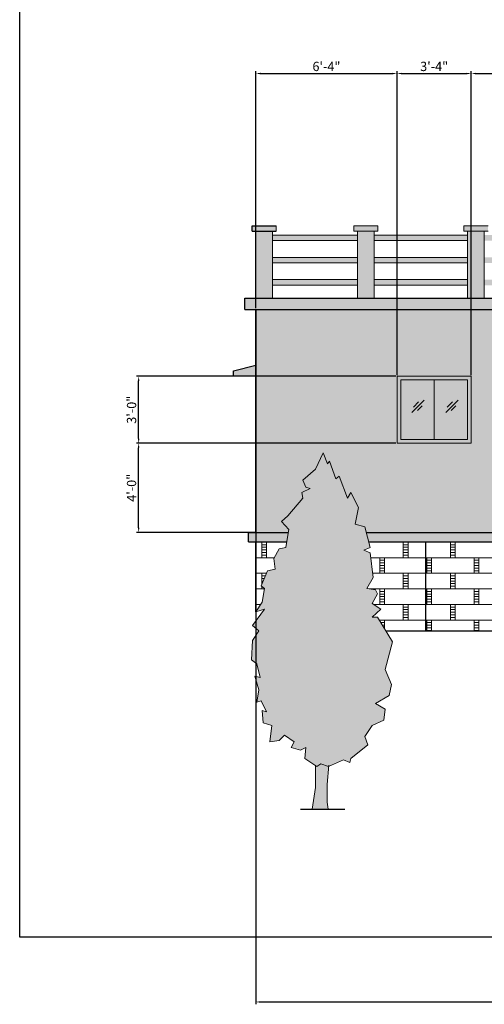
# Model space of a CAD drawing. Units: inches. Extents: x 1662 to 23131, y 1265 to 19127.
# Tile 21 of 26: x 21861 to 22111, y 17831 to 18361. Entities that reach past the tile are written whole.
import ezdxf

# ---------------------------------------------------------------- set-up
doc = ezdxf.new("R2010")
doc.units = ezdxf.units.IN
for name, color, linetype, lineweight in [('A-ANNO-DIMS', 4, 'Continuous', 18), ('A-ANNO-TTLB', 7, 'Continuous', 25), ('A-ELEV', 7, 'Continuous', 25), ('A-ELEV-GLAZ', 4, 'Continuous', 18), ('A-ELEV-PATT', 8, 'Continuous', 13), ('A-ELEV-RAIL', 7, 'Continuous', 18), ('A-ELEV-SURF-PATT', 252, 'Continuous', 13), ('L-PLNT', 3, 'Continuous', 18)]:
    doc.layers.add(name, color=color, linetype=linetype, lineweight=lineweight)
doc.styles.get("Standard").update_dxf_attribs({"font": 'arial.ttf'})
doc.dimstyles.new('ISO-25', dxfattribs={"dimtxt": 5, "dimasz": 2.5, "dimexe": 1.25, "dimexo": 0.625, "dimtad": 1, "dimlunit": 3, "dimtxsty": 'Standard', "dimcen": 2.5, "dimadec": 0, "dimazin": 0, "dimtfac": 1, "dimtmove": 0, "dimatfit": 3, "dimfxl": 1, "dimarcsym": 0})

# ---------------------------------------------------------------- blocks, each defined once
blk = doc.blocks.new('*U136')
blk.add_lwpolyline([(-69.9516, 4869.1546), (-172.212, 4644.4154), (-347.5228, 4494.6062), (-303.6824, 4400.9564), (-245.2624, 4382.2366), (-362.1278, 4326.0518), (-347.5228, 4251.1472), (-552.0182, 4007.6882), (-639.6736, 3932.7836), (-537.4132, 3820.414), (-552.0182, 3745.5094), (-581.2536, 3576.955), (-668.8836, 3558.2098), (-741.934, 3427.1204), (-727.329, 3277.3112), (-829.5894, 3258.5914), (-917.2194, 3052.572), (-873.4044, 3015.1324), (-902.6144, 2827.8582), (-990.2698, 2696.7434), (-873.4044, 2734.2084), (-1034.0848, 2509.4692), (-946.4294, 2434.5646), (-1034.0848, 2303.4752), (-1048.6898, 2041.2964), (-975.6648, 1985.1116), (-931.8244, 1797.8374), (-1004.8748, 1816.5572), (-946.4294, 1629.283), (-975.6648, 1460.7286), (-917.2194, 1479.4738), (-844.1944, 1329.6392), (-902.6144, 1348.3844), (-888.0094, 1179.83), (-771.144, 1142.365), (-800.354, 917.6512), (-668.8836, 936.371), (-595.8586, 1011.2756), (-464.3882, 917.6512), (-508.2032, 842.7212), (-376.7328, 805.2816), (-303.6824, 842.7212), (-318.2874, 692.912), (-157.607, 580.5424), (-99.187, 618.0074), (3.0734, 580.5424), (207.5942, 674.1922), (295.2496, 636.7272), (309.8546, 692.912), (543.56, 880.1862), (499.745, 992.5558), (602.0054, 1142.365), (762.6858, 1217.2696), (777.2908, 1367.1042), (645.8204, 1442.0088), (835.7362, 1554.3784), (864.9462, 1704.1876), (777.2908, 1910.207), (879.5512, 2284.7554), (675.0304, 2621.8388), (602.0054, 2621.8388), (718.8708, 2734.2084), (602.0054, 2809.113), (675.0304, 2940.2024), (645.8204, 2996.3872), (528.955, 3015.1324), (616.6104, 3164.9416), (572.7954, 3502.0504), (485.14, 3539.49), (572.7954, 3576.955), (499.745, 3857.8536), (368.2746, 3895.3186), (412.0896, 4120.0578), (309.8546, 4326.0518), (266.0142, 4251.1472), (149.1488, 4550.791), (105.3338, 4513.326), (17.6784, 4756.785), (-11.5316, 4719.32)], close=True)
for points in [[(-173.0502, 601.1926), (-173.0502, 296.3926), (-219.1258, 0)], [(9.8298, 601.1926), (-14.6304, 337.0834), (-14.6304, 93.6244), (0, 0)]]:
    blk.add_lwpolyline(points)
blk = doc.blocks.new('GLAZ-REFLECTION')
for p, q in [((0, 0), (6.63, 6.69)), ((0.83, 2.91), (3.6, 5.77)), ((2.93, 0.98), (5.5, 3.58))]:
    blk.add_line(p, q)
blk = doc.blocks.new('*D257')
at = {"layer": 'A-ANNO-DIMS', "color": 0, "lineweight": -2, "transparency": 16777216}
for p, q in [((21988.15, 18204.6), (21988.15, 17831.29)), ((22540.15, 18204.6), (22540.15, 17831.29)), ((21990.65, 17832.54), (22537.65, 17832.54))]:
    blk.add_line(p, q, dxfattribs=at)
at = {"layer": 'A-ANNO-DIMS', "color": 0, "transparency": 16777216}
for points in [[(21990.65, 17832.96), (21990.65, 17832.12), (21988.15, 17832.54)], [(22537.65, 17832.96), (22537.65, 17832.12), (22540.15, 17832.54)]]:
    blk.add_solid(points, dxfattribs=at)
at = {"layer": 'Defpoints', "color": 0, "transparency": 16777216}
for p in [(21988.15, 18205.22), (22540.15, 18205.22), (22540.15, 17832.54)]:
    blk.add_point(p, dxfattribs=at)
at = {"layer": 'A-ANNO-DIMS', "color": 0, "transparency": 16777216, "insert": (22264.15, 17835.72), "char_height": 5, "attachment_point": 5}
blk.add_mtext('46\'-0"', dxfattribs=at)
blk = doc.blocks.new('*D259')
at = {"layer": 'A-ANNO-DIMS', "color": 0, "lineweight": -2, "transparency": 16777216}
for p, q in [((21988.15, 18205.85), (21988.15, 18333.37)), ((21990.65, 18332.12), (22061.65, 18332.12)), ((22064.15, 18169.85), (22064.15, 18333.37))]:
    blk.add_line(p, q, dxfattribs=at)
at = {"layer": 'A-ANNO-DIMS', "color": 0, "transparency": 16777216}
for points in [[(21990.65, 18332.54), (21990.65, 18331.71), (21988.15, 18332.12)], [(22061.65, 18332.54), (22061.65, 18331.71), (22064.15, 18332.12)]]:
    blk.add_solid(points, dxfattribs=at)
at = {"layer": 'Defpoints', "color": 0, "transparency": 16777216}
for p in [(22064.15, 18332.12), (21988.15, 18205.22), (22064.15, 18169.22)]:
    blk.add_point(p, dxfattribs=at)
at = {"layer": 'A-ANNO-DIMS', "color": 0, "transparency": 16777216, "insert": (22026.15, 18335.3), "char_height": 5, "attachment_point": 5}
blk.add_mtext('6\'-4"', dxfattribs=at)
blk = doc.blocks.new('*D260')
at = {"layer": 'A-ANNO-DIMS', "color": 0, "lineweight": -2, "transparency": 16777216}
for p, q in [((22064.15, 18169.85), (22064.15, 18333.37)), ((22066.65, 18332.12), (22101.65, 18332.12)), ((22104.15, 18169.85), (22104.15, 18333.37))]:
    blk.add_line(p, q, dxfattribs=at)
at = {"layer": 'A-ANNO-DIMS', "color": 0, "transparency": 16777216}
for points in [[(22066.65, 18332.54), (22066.65, 18331.71), (22064.15, 18332.12)], [(22101.65, 18332.54), (22101.65, 18331.71), (22104.15, 18332.12)]]:
    blk.add_solid(points, dxfattribs=at)
at = {"layer": 'Defpoints', "color": 0, "transparency": 16777216}
for p in [(22104.15, 18332.12), (22064.15, 18169.22), (22104.15, 18169.22)]:
    blk.add_point(p, dxfattribs=at)
at = {"layer": 'A-ANNO-DIMS', "color": 0, "transparency": 16777216, "insert": (22084.15, 18335.3), "char_height": 5, "attachment_point": 5}
blk.add_mtext('3\'-4"', dxfattribs=at)
blk = doc.blocks.new('*D261')
at = {"layer": 'A-ANNO-DIMS', "color": 0, "lineweight": -2, "transparency": 16777216}
for p, q in [((22104.15, 18169.85), (22104.15, 18333.37)), ((22106.65, 18332.12), (22168.65, 18332.12)), ((22171.15, 18169.85), (22171.15, 18333.37))]:
    blk.add_line(p, q, dxfattribs=at)
at = {"layer": 'A-ANNO-DIMS', "color": 0, "transparency": 16777216}
for points in [[(22106.65, 18332.54), (22106.65, 18331.71), (22104.15, 18332.12)], [(22168.65, 18332.54), (22168.65, 18331.71), (22171.15, 18332.12)]]:
    blk.add_solid(points, dxfattribs=at)
at = {"layer": 'Defpoints', "color": 0, "transparency": 16777216}
for p in [(22171.15, 18332.12), (22104.15, 18169.22), (22171.15, 18169.22)]:
    blk.add_point(p, dxfattribs=at)
at = {"layer": 'A-ANNO-DIMS', "color": 0, "transparency": 16777216, "insert": (22137.65, 18335.29), "char_height": 5, "attachment_point": 5}
blk.add_mtext('5\'-7"', dxfattribs=at)
blk = doc.blocks.new('*D266')
at = {"layer": 'A-ANNO-DIMS', "color": 0, "lineweight": -2, "transparency": 16777216}
for p, q in [((22063.52, 18169.22), (21923.8, 18169.22)), ((21925.05, 18135.72), (21925.05, 18166.72)), ((22063.52, 18133.22), (21923.8, 18133.22))]:
    blk.add_line(p, q, dxfattribs=at)
at = {"layer": 'A-ANNO-DIMS', "color": 0, "transparency": 16777216}
for points in [[(21924.63, 18166.72), (21925.47, 18166.72), (21925.05, 18169.22)], [(21924.63, 18135.72), (21925.47, 18135.72), (21925.05, 18133.22)]]:
    blk.add_solid(points, dxfattribs=at)
at = {"layer": 'Defpoints', "color": 0, "transparency": 16777216}
for p in [(21925.05, 18169.22), (22064.15, 18169.22), (22064.15, 18133.22)]:
    blk.add_point(p, dxfattribs=at)
at = {"layer": 'A-ANNO-DIMS', "color": 0, "transparency": 16777216, "insert": (21921.87, 18151.22), "char_height": 5, "attachment_point": 5, "rotation": 90}
blk.add_mtext('3\'-0"', dxfattribs=at)
blk = doc.blocks.new('*D267')
at = {"layer": 'A-ANNO-DIMS', "color": 0, "lineweight": -2, "transparency": 16777216}
for p, q in [((22063.52, 18133.22), (21923.8, 18133.22)), ((21925.05, 18087.72), (21925.05, 18130.72)), ((21987.52, 18085.22), (21923.8, 18085.22))]:
    blk.add_line(p, q, dxfattribs=at)
at = {"layer": 'A-ANNO-DIMS', "color": 0, "transparency": 16777216}
for points in [[(21924.63, 18130.72), (21925.47, 18130.72), (21925.05, 18133.22)], [(21924.63, 18087.72), (21925.47, 18087.72), (21925.05, 18085.22)]]:
    blk.add_solid(points, dxfattribs=at)
at = {"layer": 'Defpoints', "color": 0, "transparency": 16777216}
for p in [(21925.05, 18133.22), (22064.15, 18133.22), (21988.15, 18085.22)]:
    blk.add_point(p, dxfattribs=at)
at = {"layer": 'A-ANNO-DIMS', "color": 0, "transparency": 16777216, "insert": (21921.87, 18109.22), "char_height": 5, "attachment_point": 5, "rotation": 90}
blk.add_mtext('4\'-0"', dxfattribs=at)

msp = doc.modelspace()

# ---------------------------------------------------------------- hatches: boundary and pattern name
at = {"layer": 'A-ELEV-PATT'}
h = msp.add_hatch(dxfattribs=at)
h.set_pattern_fill('BRSTONE', color=256)
h.paths.add_polyline_path([(22156.149, 18080.223), (22079.649, 18080.223), (22079.649, 18032.223), (22156.149, 18032.223)])
h.paths.add_polyline_path([(22079.649, 18080.223), (22048.849, 18080.223), (22049.648, 18077.151), (22046.197, 18075.676), (22049.648, 18074.202), (22051.373, 18060.93), (22047.922, 18055.032), (22052.523, 18054.294), (22053.673, 18052.082), (22050.798, 18046.921), (22055.399, 18043.972), (22050.798, 18039.548), (22053.673, 18039.548), (22058.118, 18032.223), (22079.649, 18032.223)])
h.paths.add_polyline_path([(21997.887, 18071.252), (22000.763, 18076.413), (22004.213, 18077.151), (22004.746, 18080.223), (21988.149, 18080.223), (21988.149, 18042.556), (21991.561, 18047.659), (21992.711, 18055.032), (21990.986, 18056.506), (21994.436, 18064.617), (21998.462, 18065.354)])
at = {"layer": 'A-ELEV-SURF-PATT'}
h = msp.add_hatch(color=256, dxfattribs=at)
h.dxf.hatch_style = 1
h.paths.add_polyline_path([(22225.149, 18211.223), (21982.149, 18211.223), (21982.149, 18205.223), (22225.149, 18205.223)])
h.paths.add_polyline_path([(22546.149, 18211.223), (22339.149, 18211.223), (22339.149, 18205.223), (22546.149, 18205.223)])
h.paths.add_polyline_path([(22351.149, 18300.223), (22213.149, 18300.223), (22213.149, 18295.223), (22351.149, 18295.223)])
h = msp.add_hatch(color=256, dxfattribs=at)
h.dxf.hatch_style = 1
h.paths.add_polyline_path([(22225.149, 18205.223), (21988.149, 18205.223), (21988.149, 18085.223), (22005.644, 18085.223), (22005.939, 18086.736), (22001.913, 18091.16), (22005.364, 18094.109), (22013.415, 18103.694), (22012.84, 18106.643), (22017.441, 18108.855), (22015.141, 18109.592), (22013.415, 18113.279), (22020.317, 18119.177), (22024.343, 18128.025), (22026.643, 18122.126), (22027.793, 18123.601), (22031.244, 18114.016), (22032.969, 18115.491), (22037.57, 18103.694), (22039.296, 18106.643), (22043.321, 18098.533), (22041.596, 18089.685), (22046.772, 18088.21), (22047.549, 18085.223), (22171.149, 18085.223), (22171.149, 18169.223), (22213.149, 18169.223), (22213.149, 18085.223), (22225.149, 18085.223)])
h.paths.add_polyline_path([(22064.149, 18169.223), (22104.149, 18169.223), (22104.149, 18133.223), (22064.149, 18133.223)], flags=16)
h.paths.add_polyline_path([(22066.149, 18167.223), (22102.149, 18167.223), (22102.149, 18135.223), (22066.149, 18135.223)], flags=0)
h.paths.add_polyline_path([(22540.149, 18205.223), (22339.149, 18205.223), (22339.149, 18085.223), (22540.149, 18085.223)])
h.paths.add_polyline_path([(22415.149, 18169.223), (22455.149, 18169.223), (22455.149, 18133.223), (22415.149, 18133.223)], flags=16)
h.paths.add_polyline_path([(22417.149, 18167.223), (22453.149, 18167.223), (22453.149, 18135.223), (22417.149, 18135.223)], flags=0)
h.paths.add_polyline_path([(22339.149, 18205.223), (22339.149, 18268.223), (22252.149, 18268.223), (22252.149, 18211.223), (22252.149, 18085.223), (22339.149, 18085.223)], flags=17)
h.paths.add_polyline_path([(22272.061, 18145.984), (22272.061, 18250.207), (22312.36, 18250.207), (22312.36, 18145.984)], flags=16)
h.paths.add_polyline_path([(22275.061, 18148.984), (22275.061, 18247.207), (22309.36, 18247.207), (22309.36, 18148.984)], flags=0)
h.paths.add_polyline_path([(22243.149, 18211.223), (22243.149, 18277.223), (22339.149, 18277.223), (22339.149, 18295.223), (22225.149, 18295.223), (22225.149, 18211.223), (22225.149, 18085.223), (22243.149, 18085.223)])
h = msp.add_hatch(color=256, dxfattribs=at)
h.dxf.hatch_style = 1
h.paths.add_polyline_path([(21999.149, 18250.223), (21986.149, 18250.223), (21986.149, 18247.223), (21999.149, 18247.223)])
h.paths.add_polyline_path([(22053.899, 18250.223), (22040.899, 18250.223), (22040.899, 18247.223), (22053.899, 18247.223)])
h.paths.add_polyline_path([(22113.149, 18250.223), (22100.149, 18250.223), (22100.149, 18247.223), (22113.149, 18247.223)])
h.paths.add_polyline_path([(22172.399, 18250.223), (22159.399, 18250.223), (22159.399, 18247.223), (22172.399, 18247.223)])
h.paths.add_polyline_path([(22363.649, 18250.223), (22350.649, 18250.223), (22350.649, 18247.223), (22363.649, 18247.223)])
h.paths.add_polyline_path([(22436.399, 18250.223), (22423.399, 18250.223), (22423.399, 18247.223), (22436.399, 18247.223)])
h.paths.add_polyline_path([(22495.649, 18250.223), (22482.649, 18250.223), (22482.649, 18247.223), (22495.649, 18247.223)])
h.paths.add_polyline_path([(22542.149, 18250.223), (22529.149, 18250.223), (22529.149, 18247.223), (22542.149, 18247.223)])
h = msp.add_hatch(color=256, dxfattribs=at)
h.dxf.hatch_style = 1
h.paths.add_polyline_path([(22493.649, 18247.223), (22484.649, 18247.223), (22484.649, 18211.223), (22493.649, 18211.223)])
h.paths.add_polyline_path([(22434.399, 18247.223), (22425.399, 18247.223), (22425.399, 18211.223), (22434.399, 18211.223)])
h.paths.add_polyline_path([(22361.649, 18247.223), (22352.649, 18247.223), (22352.649, 18211.223), (22361.649, 18211.223)])
h.paths.add_polyline_path([(22170.399, 18247.223), (22161.399, 18247.223), (22161.399, 18211.223), (22170.399, 18211.223)])
h.paths.add_polyline_path([(22111.149, 18247.223), (22102.149, 18247.223), (22102.149, 18211.223), (22111.149, 18211.223)])
h.paths.add_polyline_path([(22051.899, 18247.223), (22042.899, 18247.223), (22042.899, 18211.223), (22051.899, 18211.223)])
h.paths.add_polyline_path([(21997.149, 18247.223), (21988.149, 18247.223), (21988.149, 18211.223), (21997.149, 18211.223)])
h = msp.add_hatch(color=256, dxfattribs=at)
h.dxf.hatch_style = 1
h.paths.add_polyline_path([(22104.149, 18169.223), (22064.149, 18169.223), (22064.149, 18133.223), (22104.149, 18133.223)])
h.paths.add_polyline_path([(22102.149, 18167.223), (22102.149, 18135.223), (22066.149, 18135.223), (22066.149, 18167.223)], flags=16)
h.paths.add_polyline_path([(22455.149, 18169.223), (22415.149, 18169.223), (22415.149, 18133.223), (22455.149, 18133.223)])
h.paths.add_polyline_path([(22453.149, 18167.223), (22453.149, 18135.223), (22417.149, 18135.223), (22417.149, 18167.223)], flags=16)
h.paths.add_polyline_path([(22312.36, 18250.207), (22272.061, 18250.207), (22272.061, 18145.984), (22312.36, 18145.984)])
h.paths.add_polyline_path([(22309.36, 18148.984), (22275.061, 18148.984), (22275.061, 18247.207), (22309.36, 18247.207)], flags=16)
h.paths.add_polyline_path([(22042.899, 18245.223), (21997.149, 18245.223), (21997.149, 18242.223), (22042.899, 18242.223)])
h.paths.add_polyline_path([(22042.899, 18233.223), (21997.149, 18233.223), (21997.149, 18230.223), (22042.899, 18230.223)])
h.paths.add_polyline_path([(22042.899, 18221.223), (21997.149, 18221.223), (21997.149, 18218.223), (22042.899, 18218.223)])
h.paths.add_polyline_path([(22102.149, 18221.223), (22051.899, 18221.223), (22051.899, 18218.223), (22102.149, 18218.223)])
h.paths.add_polyline_path([(22102.149, 18233.223), (22051.899, 18233.223), (22051.899, 18230.223), (22102.149, 18230.223)])
h.paths.add_polyline_path([(22102.149, 18245.223), (22051.899, 18245.223), (22051.899, 18242.223), (22102.149, 18242.223)])
h.paths.add_polyline_path([(22161.399, 18245.223), (22111.149, 18245.223), (22111.149, 18242.223), (22161.399, 18242.223)])
h.paths.add_polyline_path([(22161.399, 18233.223), (22111.149, 18233.223), (22111.149, 18230.223), (22161.399, 18230.223)])
h.paths.add_polyline_path([(22161.399, 18221.223), (22111.149, 18221.223), (22111.149, 18218.223), (22161.399, 18218.223)])
h.paths.add_polyline_path([(22225.149, 18221.223), (22170.399, 18221.223), (22170.399, 18218.223), (22225.149, 18218.223)])
h.paths.add_polyline_path([(22225.149, 18233.223), (22170.399, 18233.223), (22170.399, 18230.223), (22225.149, 18230.223)])
h.paths.add_polyline_path([(22225.149, 18245.223), (22170.399, 18245.223), (22170.399, 18242.223), (22225.149, 18242.223)])
h.paths.add_polyline_path([(22352.649, 18233.223), (22339.149, 18233.223), (22339.149, 18230.223), (22352.649, 18230.223)])
h.paths.add_polyline_path([(22352.649, 18221.223), (22339.149, 18221.223), (22339.149, 18218.223), (22352.649, 18218.223)])
h.paths.add_polyline_path([(22352.649, 18245.223), (22339.149, 18245.223), (22339.149, 18242.223), (22352.649, 18242.223)])
h.paths.add_polyline_path([(22425.399, 18245.223), (22361.649, 18245.223), (22361.649, 18242.223), (22425.399, 18242.223)])
h.paths.add_polyline_path([(22425.399, 18233.223), (22361.649, 18233.223), (22361.649, 18230.223), (22425.399, 18230.223)])
h.paths.add_polyline_path([(22425.399, 18221.223), (22361.649, 18221.223), (22361.649, 18218.223), (22425.399, 18218.223)])
h.paths.add_polyline_path([(22484.649, 18245.223), (22434.399, 18245.223), (22434.399, 18242.223), (22484.649, 18242.223)])
h.paths.add_polyline_path([(22484.649, 18233.223), (22434.399, 18233.223), (22434.399, 18230.223), (22484.649, 18230.223)])
h.paths.add_polyline_path([(22484.649, 18221.223), (22434.399, 18221.223), (22434.399, 18218.223), (22484.649, 18218.223)])
h.paths.add_polyline_path([(22531.149, 18221.223), (22493.649, 18221.223), (22493.649, 18218.223), (22531.149, 18218.223)])
h.paths.add_polyline_path([(22531.149, 18233.223), (22493.649, 18233.223), (22493.649, 18230.223), (22531.149, 18230.223)])
h.paths.add_polyline_path([(22531.149, 18245.223), (22493.649, 18245.223), (22493.649, 18242.223), (22531.149, 18242.223)])
h = msp.add_hatch(color=256, dxfattribs=at)
h.dxf.hatch_style = 1
h.paths.add_polyline_path([(21988.149, 18175.223), (21976.149, 18172.223), (21976.149, 18169.223), (21988.149, 18169.223)])
h = msp.add_hatch(color=256, dxfattribs=at)
h.dxf.hatch_style = 1
h.paths.add_polyline_path([(22084.149, 18167.223), (22066.149, 18167.223), (22066.149, 18135.223), (22084.149, 18135.223)])
h.paths.add_polyline_path([(22102.149, 18167.223), (22084.149, 18167.223), (22084.149, 18135.223), (22102.149, 18135.223)])
h.paths.add_polyline_path([(22435.149, 18167.223), (22417.149, 18167.223), (22417.149, 18135.223), (22435.149, 18135.223)])
h.paths.add_polyline_path([(22453.149, 18167.223), (22435.149, 18167.223), (22435.149, 18135.223), (22453.149, 18135.223)])
h = msp.add_hatch(color=256, dxfattribs=at)
h.dxf.hatch_style = 1
h.paths.add_polyline_path([(22053.673, 18039.548), (22050.798, 18039.548), (22055.399, 18043.972), (22050.798, 18046.921), (22053.673, 18052.082), (22052.523, 18054.294), (22047.922, 18055.032), (22051.373, 18060.93), (22049.648, 18074.202), (22046.197, 18075.676), (22049.648, 18077.151), (22046.772, 18088.21), (22041.596, 18089.685), (22043.321, 18098.533), (22039.296, 18106.643), (22037.57, 18103.694), (22032.969, 18115.491), (22031.244, 18114.016), (22027.793, 18123.601), (22026.643, 18122.126), (22024.343, 18128.025), (22020.317, 18119.177), (22013.415, 18113.279), (22015.141, 18109.592), (22017.441, 18108.855), (22012.84, 18106.643), (22013.415, 18103.694), (22005.364, 18094.109), (22001.913, 18091.16), (22005.939, 18086.736), (22005.364, 18083.787), (22004.213, 18077.151), (22000.763, 18076.413), (21997.887, 18071.252), (21998.462, 18065.354), (21994.436, 18064.617), (21990.986, 18056.506), (21992.711, 18055.032), (21991.561, 18047.659), (21988.149, 18042.556), (21988.149, 18042.51), (21992.711, 18043.972), (21986.385, 18035.124), (21989.836, 18032.175), (21986.385, 18027.014), (21985.81, 18016.692), (21988.685, 18014.48), (21990.411, 18007.107), (21987.535, 18007.844), (21989.836, 18000.471), (21988.685, 17993.835), (21990.986, 17994.573), (21993.861, 17988.674), (21991.561, 17989.412), (21992.136, 17982.776), (21996.737, 17981.301), (21995.587, 17972.454), (22000.763, 17973.191), (22003.638, 17976.14), (22008.814, 17972.454), (22007.089, 17969.504), (22012.265, 17968.03), (22015.141, 17969.504), (22014.566, 17963.606), (22020.892, 17959.182), (22023.192, 17960.657), (22027.218, 17959.182), (22035.27, 17962.869), (22038.721, 17961.394), (22039.296, 17963.606), (22048.497, 17970.979), (22046.772, 17975.403), (22050.798, 17981.301), (22057.124, 17984.25), (22057.699, 17990.149), (22052.523, 17993.098), (22060, 17997.522), (22061.15, 18003.42), (22057.699, 18011.531), (22061.725, 18026.277)], flags=17)
h.paths.add_polyline_path([(22061.725, 18026.277), (22053.673, 18039.548), (22050.798, 18039.548), (22055.399, 18043.972), (22050.798, 18046.921), (22053.673, 18052.082), (22052.523, 18054.294), (22047.922, 18055.032), (22051.373, 18060.93), (22049.648, 18074.202), (22046.197, 18075.676), (22049.648, 18077.151), (22046.772, 18088.21), (22041.596, 18089.685), (22043.321, 18098.533), (22039.296, 18106.643), (22037.57, 18103.694), (22032.969, 18115.491), (22031.244, 18114.016), (22027.793, 18123.601), (22026.643, 18122.126), (22024.343, 18128.025), (22020.317, 18119.177), (22013.415, 18113.279), (22015.141, 18109.592), (22017.441, 18108.855), (22012.84, 18106.643), (22013.415, 18103.694), (22005.364, 18094.109), (22001.913, 18091.16), (22005.939, 18086.736), (22005.364, 18083.787), (22004.213, 18077.151), (22000.763, 18076.413), (21997.887, 18071.252), (21998.462, 18065.354), (21994.436, 18064.617), (21990.986, 18056.506), (21992.711, 18055.032), (21991.561, 18047.659), (21988.11, 18042.497), (21992.711, 18043.972), (21986.385, 18035.124), (21989.836, 18032.175), (21986.385, 18027.014), (21985.81, 18016.692), (21988.685, 18014.48), (21990.411, 18007.107), (21987.535, 18007.844), (21989.836, 18000.471), (21988.685, 17993.835), (21990.986, 17994.573), (21993.861, 17988.674), (21991.561, 17989.412), (21992.136, 17982.776), (21996.737, 17981.301), (21995.587, 17972.454), (22000.763, 17973.191), (22003.638, 17976.14), (22008.814, 17972.454), (22007.089, 17969.504), (22012.265, 17968.03), (22015.141, 17969.504), (22014.566, 17963.606), (22020.892, 17959.182), (22023.192, 17960.657), (22027.218, 17959.182), (22035.27, 17962.869), (22038.721, 17961.394), (22039.296, 17963.606), (22048.497, 17970.979), (22046.772, 17975.403), (22050.798, 17981.301), (22057.124, 17984.25), (22057.699, 17990.149), (22052.523, 17993.098), (22060, 17997.522), (22061.15, 18003.42), (22057.699, 18011.531)], flags=17)
h = msp.add_hatch(color=256, dxfattribs=at)
h.dxf.hatch_style = 1
h.paths.add_polyline_path([(22057.699, 18011.531), (22061.725, 18026.277), (22053.673, 18039.548), (22050.798, 18039.548), (22055.399, 18043.972), (22050.798, 18046.921), (22053.673, 18052.082), (22052.523, 18054.294), (22047.922, 18055.032), (22051.373, 18060.93), (22049.648, 18074.202), (22046.197, 18075.676), (22049.648, 18077.151), (22046.772, 18088.21), (22041.596, 18089.685), (22043.321, 18098.533), (22039.296, 18106.643), (22037.57, 18103.694), (22032.969, 18115.491), (22031.244, 18114.016), (22027.793, 18123.601), (22026.643, 18122.126), (22024.343, 18128.025), (22020.317, 18119.177), (22013.415, 18113.279), (22015.141, 18109.592), (22017.441, 18108.855), (22012.84, 18106.643), (22013.415, 18103.694), (22005.364, 18094.109), (22001.913, 18091.16), (22005.939, 18086.736), (22005.364, 18083.787), (22004.213, 18077.151), (22000.763, 18076.413), (21997.887, 18071.252), (21998.462, 18065.354), (21994.436, 18064.617), (21990.986, 18056.506), (21992.711, 18055.032), (21991.561, 18047.659), (21988.149, 18042.556), (21988.149, 18042.51), (21992.711, 18043.972), (21986.385, 18035.124), (21989.836, 18032.175), (21986.385, 18027.014), (21985.81, 18016.692), (21988.685, 18014.48), (21990.411, 18007.107), (21987.535, 18007.844), (21989.836, 18000.471), (21988.685, 17993.835), (21990.986, 17994.573), (21993.861, 17988.674), (21991.561, 17989.412), (21992.136, 17982.776), (21996.737, 17981.301), (21995.587, 17972.454), (22000.763, 17973.191), (22003.638, 17976.14), (22008.814, 17972.454), (22007.089, 17969.504), (22012.265, 17968.03), (22015.141, 17969.504), (22014.566, 17963.606), (22020.892, 17959.182), (22023.192, 17960.657), (22027.218, 17959.182), (22035.27, 17962.869), (22038.721, 17961.394), (22039.296, 17963.606), (22048.497, 17970.979), (22046.772, 17975.403), (22050.798, 17981.301), (22057.124, 17984.25), (22057.699, 17990.149), (22052.523, 17993.098), (22060, 17997.522), (22061.15, 18003.42)])
h = msp.add_hatch(color=256, dxfattribs=at)
h.dxf.hatch_style = 1
h.paths.add_polyline_path([(22544.149, 18085.223), (22047.549, 18085.223), (22048.849, 18080.223), (22544.149, 18080.223)])
h.paths.add_polyline_path([(22005.364, 18083.787), (22005.644, 18085.223), (21984.149, 18085.223), (21984.149, 18080.223), (22004.746, 18080.223)])
h = msp.add_hatch(color=256, dxfattribs=at)
h.dxf.hatch_style = 1
h.paths.add_polyline_path([(22026.521, 17949.597), (22027.417, 17959.274), (22027.218, 17959.182), (22023.192, 17960.657), (22020.892, 17959.182), (22020.284, 17959.608), (22020.284, 17947.995), (22018.47, 17936.326), (22027.097, 17936.326), (22026.521, 17940.012)])

# ---------------------------------------------------------------- linework, layer by layer
at = {"layer": 'A-ANNO-TTLB'}
msp.add_lwpolyline([(21860.989, 19103.605), (23130.86, 19103.605), (23130.86, 17867.351), (21860.989, 17867.351)], close=True, dxfattribs=at)
at = {"layer": 'A-ELEV'}
for p, q in [((21986.149, 18250.223), (21999.149, 18250.223)), ((21986.149, 18247.223), (21986.149, 18250.223)), ((21986.149, 18247.223), (21999.149, 18247.223)), ((21982.149, 18211.223), (22225.149, 18211.223)), ((21982.149, 18205.223), (21982.149, 18211.223)), ((21982.149, 18205.223), (22225.149, 18205.223)), ((21988.149, 18085.223), (21988.149, 18205.223)), ((21976.149, 18172.223), (21988.149, 18175.223)), ((21988.149, 18169.223), (21988.149, 18175.223)), ((21976.149, 18169.223), (21976.149, 18172.223)), ((21988.149, 18169.223), (21976.149, 18169.223)), ((22024.343, 18128.025), (22024.343, 18128.025)), ((21984.149, 18085.223), (22005.644, 18085.223)), ((21984.149, 18080.223), (21984.149, 18085.223)), ((22047.549, 18085.223), (22544.149, 18085.223)), ((21984.149, 18080.223), (22004.746, 18080.223)), ((21988.149, 18042.51), (21988.149, 18080.223)), ((22048.849, 18080.223), (22544.149, 18080.223)), ((22079.649, 18032.223), (22079.649, 18080.223)), ((22058.118, 18032.223), (22540.149, 18032.223)), ((22012.202, 17936.326), (22036.112, 17936.326))]:
    msp.add_line(p, q, dxfattribs=at)
at = {"layer": 'A-ELEV-GLAZ'}
for p, q in [((22064.149, 18169.223), (22064.149, 18133.223)), ((22104.149, 18169.223), (22064.149, 18169.223)), ((22066.149, 18167.223), (22066.149, 18135.223)), ((22102.149, 18167.223), (22066.149, 18167.223)), ((22084.149, 18167.223), (22084.149, 18135.223)), ((22102.149, 18167.223), (22102.149, 18135.223)), ((22104.149, 18169.223), (22104.149, 18133.223)), ((22102.149, 18135.223), (22066.149, 18135.223)), ((22104.149, 18133.223), (22064.149, 18133.223))]:
    msp.add_line(p, q, dxfattribs=at)
at = {"layer": 'A-ELEV-RAIL'}
for p, q in [((21988.149, 18211.223), (21988.149, 18247.223)), ((21997.149, 18211.223), (21997.149, 18247.223)), ((21999.149, 18247.223), (21999.149, 18250.223)), ((22040.899, 18247.223), (22040.899, 18250.223)), ((22040.899, 18250.223), (22053.899, 18250.223)), ((22040.899, 18247.223), (22053.899, 18247.223)), ((22042.899, 18247.223), (22042.899, 18211.223)), ((22051.899, 18247.223), (22051.899, 18211.223)), ((22053.899, 18247.223), (22053.899, 18250.223)), ((22100.149, 18247.223), (22100.149, 18250.223)), ((22100.149, 18250.223), (22113.149, 18250.223)), ((22100.149, 18247.223), (22113.149, 18247.223)), ((22102.149, 18247.223), (22102.149, 18211.223)), ((22111.149, 18247.223), (22111.149, 18211.223)), ((21997.149, 18245.223), (22042.899, 18245.223)), ((21997.149, 18242.223), (22042.899, 18242.223)), ((22051.899, 18245.223), (22102.149, 18245.223)), ((22051.899, 18242.223), (22102.149, 18242.223)), ((21997.149, 18233.223), (22042.899, 18233.223)), ((22051.899, 18233.223), (22102.149, 18233.223)), ((21997.149, 18230.223), (22042.899, 18230.223)), ((22051.899, 18230.223), (22102.149, 18230.223)), ((21997.149, 18221.223), (22042.899, 18221.223)), ((22051.899, 18221.223), (22102.149, 18221.223)), ((21997.149, 18218.223), (22042.899, 18218.223)), ((22051.899, 18218.223), (22102.149, 18218.223))]:
    msp.add_line(p, q, dxfattribs=at)

# ---------------------------------------------------------------- block references
at = {"layer": 'A-ELEV-GLAZ'}
for p in [(22072.192, 18149.759), (22090.365, 18149.759)]:
    msp.add_blockref('GLAZ-REFLECTION', p, dxfattribs=at)
at = {"layer": 'L-PLNT', "xscale": 0.0393700787401575, "yscale": 0.0393700787401575, "zscale": 0.0393700787401575}
msp.add_blockref('*U136', (22027.097, 17936.326), dxfattribs=at)

# ---------------------------------------------------------------- dimensions: what is measured, and where the dimension line sits
at = {"layer": 'A-ANNO-DIMS'}
for base, p1, p2, picture, middle in [((22064.149, 18332.123), (21988.149, 18205.223), (22064.149, 18169.223), '*D259', (22026.149, 18335.3)), ((22104.149, 18332.123), (22064.149, 18169.223), (22104.149, 18169.223), '*D260', (22084.149, 18335.302)), ((22171.149, 18332.123), (22104.149, 18169.223), (22171.149, 18169.223), '*D261', (22137.649, 18335.29)), ((22540.149, 17832.539), (21988.149, 18205.223), (22540.149, 18205.223), '*D257', (22264.149, 17835.717))]:
    dim = msp.add_linear_dim(base=base, p1=p1, p2=p2, dimstyle='ISO-25', override={"dimdec": 1, "dimlfac": 1, "dimrnd": 0, "dimzin": 1, "dimdsep": 46, "dimlunit": 4, "dimfrac": 2}, dxfattribs=at)
    dim.commit()
    dim.dimension.update_dxf_attribs({"geometry": picture, "text_midpoint": middle})
for base, p1, p2, picture, middle in [((21925.051, 18169.223), (22064.149, 18133.223), (22064.149, 18169.223), '*D266', (21921.871, 18151.223)), ((21925.051, 18133.223), (21988.149, 18085.223), (22064.149, 18133.223), '*D267', (21921.873, 18109.223))]:
    dim = msp.add_linear_dim(base=base, p1=p1, p2=p2, angle=90, dimstyle='ISO-25', override={"dimdec": 1, "dimlfac": 1, "dimrnd": 0, "dimzin": 1, "dimdsep": 46, "dimlunit": 4, "dimfrac": 2}, dxfattribs=at)
    dim.commit()
    dim.dimension.update_dxf_attribs({"geometry": picture, "text_midpoint": middle})

doc.saveas('drawing.dxf')
